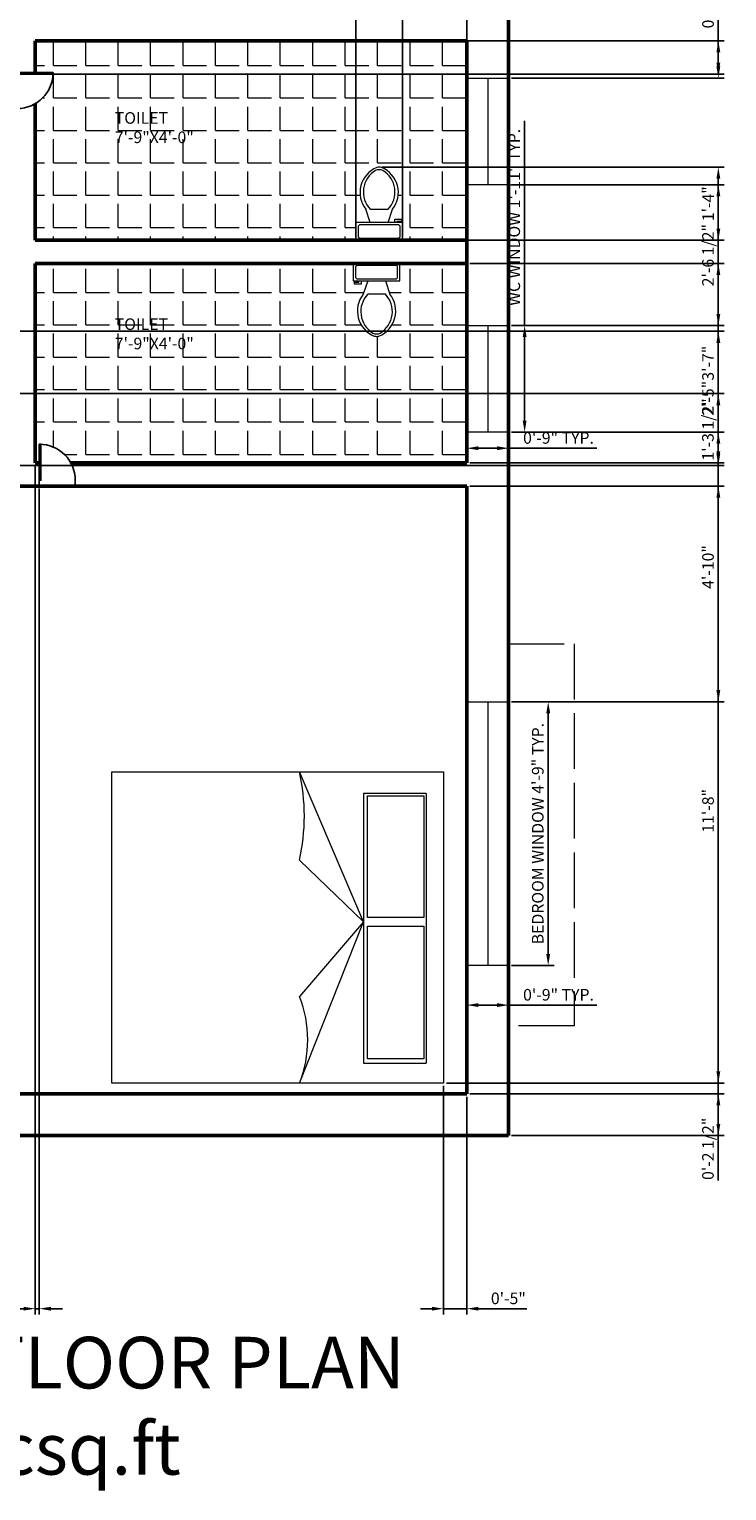
# Model space of a CAD drawing. Units: millimetres. Extents: x 3095 to 3505, y 1097 to 1734.
# Tile 3 of 5: x 3355 to 3505, y 1097 to 1412. Entities that reach past the tile are written whole.
import ezdxf

# ---------------------------------------------------------------- set-up
doc = ezdxf.new("R2010")
doc.units = ezdxf.units.MM
doc.linetypes.add('ACAD_ISO02W100', pattern=[15, 12, -3])
for name, color, linetype, lineweight, true_color in [('A-ANNO-DIMS', 32, 'Continuous', 18, 0xcd6928), ('A-ANNO-TEXT', 152, 'Continuous', 25, 0x2776bb), ('A-AREA-IDEN', 152, 'Continuous', 18, 0x2776bb), ('A-FLOR-FIXT', 9, 'Continuous', 18, 0xafd9aa), ('A-FLOR-PATT', 241, 'Continuous', 13, 0xf7abae), ('A-FURN', 9, 'Continuous', 18, 0xafd9aa), ('A-GLAZ', 9, 'Continuous', 18, 0xd19cc7), ('A-ROOF-OVHD', 152, 'ACAD_ISO02W100', 13, 0x2776bb)]:
    doc.layers.add(name, color=color, linetype=linetype, lineweight=lineweight, true_color=true_color)
doc.layers.add('A-DOOR', color=4, linetype='Continuous', lineweight=25)
doc.layers.add('A-WALL', color=7, linetype='Continuous', lineweight=50)
doc.styles.get("Standard").update_dxf_attribs({"font": 'arial.ttf'})
doc.dimstyles.new('ISO-25', dxfattribs={"dimtxt": 2.5, "dimasz": 2.5, "dimexe": 1.25, "dimexo": 0.625, "dimtad": 1, "dimlunit": 3, "dimtxsty": 'Standard', "dimcen": 2.5, "dimadec": 0, "dimazin": 0, "dimtfac": 1, "dimtmove": 0, "dimatfit": 3, "dimfxl": 1, "dimarcsym": 0})

# ---------------------------------------------------------------- blocks, each defined once
blk = doc.blocks.new('*U4')
for p, q in [((9.5, -6), (9.5, -2)), ((-10, -8.5), (-8, -8.5)), ((-10, -9.5), (-10, -8.5)), ((-7, -9.5), (-10, -9.5)), ((-8, -8.5), (-8, -8)), ((-7, -8), (-7, -9.5)), ((-4, -8), (-6, -14)), ((4, -8), (6, -14)), ((4, -14), (-4, -14))]:
    blk.add_line(p, q)
blk.add_lwpolyline([(10.5, -8), (10.5, 0), (-10.5, 0), (-10.5, -8)], close=True)
for points in [[(-9.5, -2), (-9.5, -6)], [(8.5, -1), (-8.5, -1)], [(-8.5, -7), (8.5, -7)]]:
    blk.add_lwpolyline(points)
for centre, radius, start, end in [((-8.62, -1.88), 0.884, 81.8699, 188.1301), ((-8.62, -6.12), 0.884, 171.8699, 278.1301), ((8.62, -1.88), 0.884, 351.8699, 98.1301), ((8.62, -6.12), 0.884, 261.8699, 8.1301), ((3.52, -21.58), 12.17, 141.46911, 247.97143), ((4.2, -21.82), 11.33, 136.36773, 238.94682), ((-3.52, -21.58), 12.17, 292.02843, 38.53071), ((-4.2, -21.82), 11.33, 301.05301, 43.63209), ((0, -27.88), 4, 245.73182, 294.26817), ((0, -29), 4, 254.86053, 285.13947)]:
    blk.add_arc(centre, radius, start, end)
blk = doc.blocks.new('*U8')
for p, q in [((0, 0), (0, -6)), ((40, 0), (40, -6))]:
    blk.add_line(p, q)
blk.add_lwpolyline([(0, 0), (0, 40), (1.75, 40), (1.75, 0)], close=True)
blk.add_arc((0, 0), 40, 0, 90)
blk = doc.blocks.new('*U6')
for p, q in [((0, 0), (0, -6)), ((40, 0), (40, -6))]:
    blk.add_line(p, q)
blk.add_lwpolyline([(0, 0), (0, 40), (1.75, 40), (1.75, 0)], close=True)
blk.add_arc((0, 0), 40, 0, 90)
blk = doc.blocks.new('BED-DOUBLE')
for p, q in [((4.67, 67.71), (4.67, 54.2)), ((4.67, 67.71), (62.81, 67.71)), ((62.81, 54.2), (62.81, 67.71)), ((32.4, 54.2), (0, 40.37)), ((4.67, 54.2), (62.81, 54.2)), ((32.4, 54.2), (19.1, 40.37)), ((67.13, 40.37), (32.4, 54.2)), ((32.4, 54.2), (48.47, 40.37))]:
    blk.add_line(p, q)
for points in [[(0, 71.42), (67.13, 71.42), (67.13, 0), (0, 0)], [(5.23, 67.2), (31.46, 67.2), (31.46, 55.05), (5.23, 55.05)], [(33.33, 67.2), (61.88, 67.2), (61.88, 55.05), (33.33, 55.05)]]:
    blk.add_lwpolyline(points, close=True)
for centre, radius, start, end in [((9.55, -1.59), 43.03, 77.1763, 102.8237), ((57.8, 17.19), 24.99, 68.0833, 111.9167)]:
    blk.add_arc(centre, radius, start, end)
blk = doc.blocks.new('WIN-BEDROOM')
for p, q in [((0, 56.87), (9, 56.87)), ((0, 0), (0, 56.87)), ((0, 56.87), (4.5, 56.87)), ((4.5, 56.87), (4.5, 0)), ((9, 56.87), (9, 0)), ((9, 0), (0, 0))]:
    blk.add_line(p, q)
blk = doc.blocks.new('WIN-TOILET')
for p, q in [((0, 23.01), (9, 23.01)), ((0, 0), (0, 23.01)), ((0, 23.01), (4.5, 23.01)), ((4.5, 23.01), (4.5, 0)), ((9, 23.01), (9, 0)), ((9, 0), (0, 0))]:
    blk.add_line(p, q)
blk = doc.blocks.new('*D20')
at = {"layer": 'A-ANNO-DIMS', "color": 0, "lineweight": -2, "transparency": 16777216}
for p, q in [((3458.49, 1266.84), (3467.64, 1266.84)), ((3466.39, 1212.47), (3466.39, 1264.34)), ((3458.49, 1209.97), (3467.64, 1209.97))]:
    blk.add_line(p, q, dxfattribs=at)
at = {"layer": 'A-ANNO-DIMS', "color": 0, "lineweight": 5, "transparency": 16777216}
for points in [[(3465.98, 1264.34), (3466.81, 1264.34), (3466.39, 1266.84)], [(3465.98, 1212.47), (3466.81, 1212.47), (3466.39, 1209.97)]]:
    blk.add_solid(points, dxfattribs=at)
at = {"layer": 'Defpoints', "color": 0, "lineweight": 5, "transparency": 16777216}
for p in [(3457.86, 1266.84), (3466.39, 1266.84), (3457.86, 1209.97)]:
    blk.add_point(p, dxfattribs=at)
at = {"layer": 'A-ANNO-DIMS', "color": 0, "transparency": 16777216, "insert": (3464.47, 1238.41), "char_height": 2.5, "attachment_point": 5, "rotation": 90}
blk.add_mtext('BEDROOM WINDOW 4\'-9" TYP.', dxfattribs=at)
blk = doc.blocks.new('*D21')
at = {"layer": 'A-ANNO-DIMS', "color": 0, "lineweight": -2, "transparency": 16777216}
for p, q in [((3448.86, 1209.35), (3448.86, 1200.19)), ((3457.86, 1209.35), (3457.86, 1200.19)), ((3451.36, 1201.44), (3455.36, 1201.44)), ((3457.86, 1201.44), (3476.85, 1201.44))]:
    blk.add_line(p, q, dxfattribs=at)
at = {"layer": 'A-ANNO-DIMS', "color": 0, "lineweight": 5, "transparency": 16777216}
for points in [[(3451.36, 1201.86), (3451.36, 1201.03), (3448.86, 1201.44)], [(3455.36, 1201.86), (3455.36, 1201.03), (3457.86, 1201.44)]]:
    blk.add_solid(points, dxfattribs=at)
at = {"layer": 'Defpoints', "color": 0, "lineweight": 5, "transparency": 16777216}
for p in [(3448.86, 1209.97), (3457.86, 1209.97), (3457.86, 1201.44)]:
    blk.add_point(p, dxfattribs=at)
at = {"layer": 'A-ANNO-DIMS', "color": 0, "transparency": 16777216, "insert": (3468.61, 1203.35), "char_height": 2.5, "attachment_point": 5}
blk.add_mtext('0\'-9" TYP.', dxfattribs=at)
blk = doc.blocks.new('*D22')
at = {"layer": 'A-ANNO-DIMS', "color": 0, "lineweight": -2, "transparency": 16777216}
for p, q in [((3461.31, 1347.95), (3461.31, 1392.07)), ((3458.49, 1347.95), (3462.56, 1347.95)), ((3461.31, 1327.44), (3461.31, 1345.45)), ((3458.49, 1324.94), (3462.56, 1324.94))]:
    blk.add_line(p, q, dxfattribs=at)
at = {"layer": 'A-ANNO-DIMS', "color": 0, "lineweight": 5, "transparency": 16777216}
for points in [[(3460.9, 1345.45), (3461.73, 1345.45), (3461.31, 1347.95)], [(3460.9, 1327.44), (3461.73, 1327.44), (3461.31, 1324.94)]]:
    blk.add_solid(points, dxfattribs=at)
at = {"layer": 'Defpoints', "color": 0, "lineweight": 5, "transparency": 16777216}
for p in [(3457.86, 1347.95), (3461.31, 1347.95), (3457.86, 1324.94)]:
    blk.add_point(p, dxfattribs=at)
at = {"layer": 'A-ANNO-DIMS', "color": 0, "transparency": 16777216, "insert": (3459.4, 1371.26), "char_height": 2.5, "attachment_point": 5, "rotation": 90}
blk.add_mtext('WC WINDOW 1\'-11" TYP.', dxfattribs=at)
blk = doc.blocks.new('*D23')
at = {"layer": 'A-ANNO-DIMS', "color": 0, "lineweight": -2, "transparency": 16777216}
for p, q in [((3448.86, 1324.32), (3448.86, 1320.24)), ((3457.86, 1324.32), (3457.86, 1320.24)), ((3451.36, 1321.49), (3455.36, 1321.49)), ((3457.86, 1321.49), (3476.85, 1321.49))]:
    blk.add_line(p, q, dxfattribs=at)
at = {"layer": 'A-ANNO-DIMS', "color": 0, "lineweight": 5, "transparency": 16777216}
for points in [[(3451.36, 1321.91), (3451.36, 1321.08), (3448.86, 1321.49)], [(3455.36, 1321.91), (3455.36, 1321.08), (3457.86, 1321.49)]]:
    blk.add_solid(points, dxfattribs=at)
at = {"layer": 'Defpoints', "color": 0, "lineweight": 5, "transparency": 16777216}
for p in [(3448.86, 1324.94), (3457.86, 1324.94), (3457.86, 1321.49)]:
    blk.add_point(p, dxfattribs=at)
at = {"layer": 'A-ANNO-DIMS', "color": 0, "transparency": 16777216, "insert": (3468.61, 1323.39), "char_height": 2.5, "attachment_point": 5}
blk.add_mtext('0\'-9" TYP.', dxfattribs=at)
blk = doc.blocks.new('*D40')
at = {"layer": 'A-ANNO-DIMS', "color": 0, "lineweight": -2, "transparency": 16777216}
for p, q in [((3458.49, 1454.16), (3504.29, 1454.16)), ((3503.04, 1451.66), (3503.04, 1403.79)), ((3458.49, 1401.29), (3504.29, 1401.29))]:
    blk.add_line(p, q, dxfattribs=at)
at = {"layer": 'A-ANNO-DIMS', "color": 0, "lineweight": 5, "transparency": 16777216}
for points in [[(3502.63, 1451.66), (3503.46, 1451.66), (3503.04, 1454.16)], [(3502.63, 1403.79), (3503.46, 1403.79), (3503.04, 1401.29)]]:
    blk.add_solid(points, dxfattribs=at)
at = {"layer": 'Defpoints', "color": 0, "lineweight": 5, "transparency": 16777216}
for p in [(3457.86, 1454.16), (3457.86, 1401.29), (3503.04, 1401.29)]:
    blk.add_point(p, dxfattribs=at)
at = {"layer": 'A-ANNO-DIMS', "color": 0, "transparency": 16777216, "insert": (3501.15, 1427.72), "char_height": 2.5, "attachment_point": 5, "rotation": 90}
blk.add_mtext('4\'-5"', dxfattribs=at)
blk = doc.blocks.new('*D41')
at = {"layer": 'A-ANNO-DIMS', "color": 0, "lineweight": -2, "transparency": 16777216}
for p, q in [((3458.49, 1378.28), (3504.29, 1378.28)), ((3503.04, 1375.78), (3503.04, 1350.45)), ((3458.49, 1347.95), (3504.29, 1347.95))]:
    blk.add_line(p, q, dxfattribs=at)
at = {"layer": 'A-ANNO-DIMS', "color": 0, "lineweight": 5, "transparency": 16777216}
for points in [[(3502.63, 1375.78), (3503.46, 1375.78), (3503.04, 1378.28)], [(3502.63, 1350.45), (3503.46, 1350.45), (3503.04, 1347.95)]]:
    blk.add_solid(points, dxfattribs=at)
at = {"layer": 'Defpoints', "color": 0, "lineweight": 5, "transparency": 16777216}
for p in [(3457.86, 1378.28), (3457.86, 1347.95), (3503.04, 1347.95)]:
    blk.add_point(p, dxfattribs=at)
at = {"layer": 'A-ANNO-DIMS', "color": 0, "transparency": 16777216, "insert": (3501.13, 1363.11), "char_height": 2.5, "attachment_point": 5, "rotation": 90}
blk.add_mtext('2\'-6 1/2"', dxfattribs=at)
blk = doc.blocks.new('*D42')
at = {"layer": 'A-ANNO-DIMS', "color": 0, "lineweight": -2, "transparency": 16777216}
for p, q in [((3458.49, 1324.94), (3504.29, 1324.94)), ((3503.04, 1322.44), (3503.04, 1269.34)), ((3458.49, 1266.84), (3504.29, 1266.84))]:
    blk.add_line(p, q, dxfattribs=at)
at = {"layer": 'A-ANNO-DIMS', "color": 0, "lineweight": 5, "transparency": 16777216}
for points in [[(3502.63, 1322.44), (3503.46, 1322.44), (3503.04, 1324.94)], [(3502.63, 1269.34), (3503.46, 1269.34), (3503.04, 1266.84)]]:
    blk.add_solid(points, dxfattribs=at)
at = {"layer": 'Defpoints', "color": 0, "lineweight": 5, "transparency": 16777216}
for p in [(3457.86, 1324.94), (3457.86, 1266.84), (3503.04, 1266.84)]:
    blk.add_point(p, dxfattribs=at)
at = {"layer": 'A-ANNO-DIMS', "color": 0, "transparency": 16777216, "insert": (3501.14, 1295.89), "char_height": 2.5, "attachment_point": 5, "rotation": 90}
blk.add_mtext('4\'-10"', dxfattribs=at)
blk = doc.blocks.new('*D46')
at = {"layer": 'A-ANNO-DIMS', "color": 0, "lineweight": -2, "transparency": 16777216}
for p, q in [((3449.49, 1313.32), (3504.29, 1313.32)), ((3503.04, 1310.82), (3503.04, 1175.82)), ((3458.49, 1173.32), (3504.29, 1173.32))]:
    blk.add_line(p, q, dxfattribs=at)
at = {"layer": 'A-ANNO-DIMS', "color": 0, "lineweight": 5, "transparency": 16777216}
for points in [[(3502.63, 1310.82), (3503.46, 1310.82), (3503.04, 1313.32)], [(3502.63, 1175.82), (3503.46, 1175.82), (3503.04, 1173.32)]]:
    blk.add_solid(points, dxfattribs=at)
at = {"layer": 'Defpoints', "color": 0, "lineweight": 5, "transparency": 16777216}
for p in [(3448.86, 1313.32), (3457.86, 1173.32), (3503.04, 1173.32)]:
    blk.add_point(p, dxfattribs=at)
at = {"layer": 'A-ANNO-DIMS', "color": 0, "transparency": 16777216, "insert": (3501.14, 1243.32), "char_height": 2.5, "attachment_point": 5, "rotation": 90}
blk.add_mtext('11\'-8"', dxfattribs=at)
blk = doc.blocks.new('*D47')
at = {"layer": 'A-ANNO-DIMS', "color": 0, "lineweight": -2, "transparency": 16777216}
for p, q in [((3449.49, 1361.32), (3504.29, 1361.32)), ((3503.04, 1320.82), (3503.04, 1358.82)), ((3449.49, 1318.32), (3504.29, 1318.32))]:
    blk.add_line(p, q, dxfattribs=at)
at = {"layer": 'A-ANNO-DIMS', "color": 0, "lineweight": 5, "transparency": 16777216}
for points in [[(3502.63, 1358.82), (3503.46, 1358.82), (3503.04, 1361.32)], [(3502.63, 1320.82), (3503.46, 1320.82), (3503.04, 1318.32)]]:
    blk.add_solid(points, dxfattribs=at)
at = {"layer": 'Defpoints', "color": 0, "lineweight": 5, "transparency": 16777216}
for p in [(3448.86, 1361.32), (3503.04, 1361.32), (3448.86, 1318.32)]:
    blk.add_point(p, dxfattribs=at)
at = {"layer": 'A-ANNO-DIMS', "color": 0, "transparency": 16777216, "insert": (3501.14, 1339.82), "char_height": 2.5, "attachment_point": 5, "rotation": 90}
blk.add_mtext('3\'-7"', dxfattribs=at)
blk = doc.blocks.new('*D59')
at = {"layer": 'A-ANNO-DIMS', "color": 0, "lineweight": -2, "transparency": 16777216}
for p, q in [((3424.96, 1366.94), (3424.96, 1729.27)), ((3427.46, 1728.02), (3432.49, 1728.02)), ((3434.99, 1366.94), (3434.99, 1729.27))]:
    blk.add_line(p, q, dxfattribs=at)
at = {"layer": 'A-ANNO-DIMS', "color": 0, "lineweight": 5, "transparency": 16777216}
for points in [[(3427.46, 1728.43), (3427.46, 1727.6), (3424.96, 1728.02)], [(3432.49, 1728.43), (3432.49, 1727.6), (3434.99, 1728.02)]]:
    blk.add_solid(points, dxfattribs=at)
at = {"layer": 'Defpoints', "color": 0, "lineweight": 5, "transparency": 16777216}
for p in [(3434.99, 1728.02), (3424.96, 1366.32), (3434.99, 1366.32)]:
    blk.add_point(p, dxfattribs=at)
at = {"layer": 'A-ANNO-DIMS', "color": 0, "transparency": 16777216, "insert": (3429.98, 1729.92), "char_height": 2.5, "attachment_point": 5}
blk.add_mtext('0\'-10"', dxfattribs=at)
blk = doc.blocks.new('*D60')
at = {"layer": 'A-ANNO-DIMS', "color": 0, "lineweight": -2, "transparency": 16777216}
for p, q in [((3430.6, 1382.07), (3504.29, 1382.07)), ((3503.04, 1368.82), (3503.04, 1379.57)), ((3435.62, 1366.32), (3504.29, 1366.32))]:
    blk.add_line(p, q, dxfattribs=at)
at = {"layer": 'A-ANNO-DIMS', "color": 0, "lineweight": 5, "transparency": 16777216}
for points in [[(3502.63, 1379.57), (3503.46, 1379.57), (3503.04, 1382.07)], [(3502.63, 1368.82), (3503.46, 1368.82), (3503.04, 1366.32)]]:
    blk.add_solid(points, dxfattribs=at)
at = {"layer": 'Defpoints', "color": 0, "lineweight": 5, "transparency": 16777216}
for p in [(3429.98, 1382.07), (3503.04, 1382.07), (3434.99, 1366.32)]:
    blk.add_point(p, dxfattribs=at)
at = {"layer": 'A-ANNO-DIMS', "color": 0, "transparency": 16777216, "insert": (3501.16, 1374.2), "char_height": 2.5, "attachment_point": 5, "rotation": 90}
blk.add_mtext('1\'-4"', dxfattribs=at)
blk = doc.blocks.new('*D61')
at = {"layer": 'A-ANNO-DIMS', "color": 0, "lineweight": -2, "transparency": 16777216}
for p, q in [((3434.99, 1366.94), (3434.99, 1729.27)), ((3437.49, 1728.02), (3446.36, 1728.02)), ((3448.86, 1366.94), (3448.86, 1729.27))]:
    blk.add_line(p, q, dxfattribs=at)
at = {"layer": 'A-ANNO-DIMS', "color": 0, "lineweight": 5, "transparency": 16777216}
for points in [[(3437.49, 1728.43), (3437.49, 1727.6), (3434.99, 1728.02)], [(3446.36, 1728.43), (3446.36, 1727.6), (3448.86, 1728.02)]]:
    blk.add_solid(points, dxfattribs=at)
at = {"layer": 'Defpoints', "color": 0, "lineweight": 5, "transparency": 16777216}
for p in [(3448.86, 1728.02), (3434.99, 1366.32), (3448.86, 1366.32)]:
    blk.add_point(p, dxfattribs=at)
at = {"layer": 'A-ANNO-DIMS', "color": 0, "transparency": 16777216, "insert": (3441.93, 1729.9), "char_height": 2.5, "attachment_point": 5}
blk.add_mtext('1\'-2"', dxfattribs=at)
blk = doc.blocks.new('*D63')
at = {"layer": 'A-ANNO-DIMS', "color": 0, "lineweight": -2, "transparency": 16777216}
for p, q in [((3503.04, 1409.32), (3503.04, 1419.71)), ((3356.49, 1409.32), (3504.29, 1409.32)), ((3503.04, 1404.64), (3503.04, 1406.82)), ((3356.49, 1402.14), (3504.29, 1402.14))]:
    blk.add_line(p, q, dxfattribs=at)
at = {"layer": 'A-ANNO-DIMS', "color": 0, "lineweight": 5, "transparency": 16777216}
for points in [[(3502.63, 1406.82), (3503.46, 1406.82), (3503.04, 1409.32)], [(3502.63, 1404.64), (3503.46, 1404.64), (3503.04, 1402.14)]]:
    blk.add_solid(points, dxfattribs=at)
at = {"layer": 'Defpoints', "color": 0, "lineweight": 5, "transparency": 16777216}
for p in [(3355.86, 1409.32), (3503.04, 1409.32), (3355.86, 1402.14)]:
    blk.add_point(p, dxfattribs=at)
at = {"layer": 'A-ANNO-DIMS', "color": 0, "transparency": 16777216, "insert": (3501.14, 1415.76), "char_height": 2.5, "attachment_point": 5, "rotation": 90}
blk.add_mtext('0\'-7"', dxfattribs=at)
blk = doc.blocks.new('*D64')
at = {"layer": 'A-ANNO-DIMS', "color": 0, "lineweight": -2, "transparency": 16777216}
for p, q in [((3355.86, 1317.69), (3355.86, 1134.75)), ((3356.76, 1312.81), (3356.76, 1134.75)), ((3353.36, 1136), (3342.97, 1136)), ((3356.76, 1136), (3355.86, 1136)), ((3359.26, 1136), (3361.76, 1136))]:
    blk.add_line(p, q, dxfattribs=at)
at = {"layer": 'A-ANNO-DIMS', "color": 0, "lineweight": 5, "transparency": 16777216}
for points in [[(3353.36, 1136.41), (3353.36, 1135.58), (3355.86, 1136)], [(3359.26, 1136.41), (3359.26, 1135.58), (3356.76, 1136)]]:
    blk.add_solid(points, dxfattribs=at)
at = {"layer": 'Defpoints', "color": 0, "lineweight": 5, "transparency": 16777216}
for p in [(3355.86, 1318.32), (3356.76, 1313.43), (3355.86, 1136)]:
    blk.add_point(p, dxfattribs=at)
at = {"layer": 'A-ANNO-DIMS', "color": 0, "transparency": 16777216, "insert": (3346.91, 1137.9), "char_height": 2.5, "attachment_point": 5}
blk.add_mtext('0\'-1"', dxfattribs=at)
blk = doc.blocks.new('*D69')
at = {"layer": 'A-ANNO-DIMS', "color": 0, "lineweight": -2, "transparency": 16777216}
for p, q in [((3250.48, 1333.27), (3504.29, 1333.27)), ((3503.04, 1330.77), (3503.04, 1320.3)), ((3250.48, 1317.8), (3504.29, 1317.8))]:
    blk.add_line(p, q, dxfattribs=at)
at = {"layer": 'A-ANNO-DIMS', "color": 0, "lineweight": 5, "transparency": 16777216}
for points in [[(3502.63, 1330.77), (3503.46, 1330.77), (3503.04, 1333.27)], [(3502.63, 1320.3), (3503.46, 1320.3), (3503.04, 1317.8)]]:
    blk.add_solid(points, dxfattribs=at)
at = {"layer": 'Defpoints', "color": 0, "lineweight": 5, "transparency": 16777216}
for p in [(3249.85, 1333.27), (3249.85, 1317.8), (3503.04, 1317.8)]:
    blk.add_point(p, dxfattribs=at)
at = {"layer": 'A-ANNO-DIMS', "color": 0, "transparency": 16777216, "insert": (3501.12, 1325.54), "char_height": 2.5, "attachment_point": 5, "rotation": 90}
blk.add_mtext('1\'-3 1/2"', dxfattribs=at)
blk = doc.blocks.new('*D77')
at = {"layer": 'A-ANNO-DIMS', "color": 0, "lineweight": -2, "transparency": 16777216}
for p, q in [((3194.49, 1346.71), (3504.29, 1346.71)), ((3503.04, 1344.21), (3503.04, 1320.3)), ((3250.48, 1317.8), (3504.29, 1317.8))]:
    blk.add_line(p, q, dxfattribs=at)
at = {"layer": 'A-ANNO-DIMS', "color": 0, "lineweight": 5, "transparency": 16777216}
for points in [[(3502.63, 1344.21), (3503.46, 1344.21), (3503.04, 1346.71)], [(3502.63, 1320.3), (3503.46, 1320.3), (3503.04, 1317.8)]]:
    blk.add_solid(points, dxfattribs=at)
at = {"layer": 'Defpoints', "color": 0, "lineweight": 5, "transparency": 16777216}
for p in [(3193.86, 1346.71), (3249.85, 1317.8), (3503.04, 1317.8)]:
    blk.add_point(p, dxfattribs=at)
at = {"layer": 'A-ANNO-DIMS', "color": 0, "transparency": 16777216, "insert": (3501.14, 1332.26), "char_height": 2.5, "attachment_point": 5, "rotation": 90}
blk.add_mtext('2\'-5"', dxfattribs=at)
blk = doc.blocks.new('*D86')
at = {"layer": 'A-ANNO-DIMS', "color": 0, "lineweight": -2, "transparency": 16777216}
for p, q in [((3503.04, 1187.14), (3503.04, 1189.64)), ((3444.47, 1184.64), (3504.29, 1184.64)), ((3449.49, 1182.32), (3504.29, 1182.32)), ((3503.04, 1184.64), (3503.04, 1182.32)), ((3503.04, 1179.82), (3503.04, 1163.6))]:
    blk.add_line(p, q, dxfattribs=at)
at = {"layer": 'A-ANNO-DIMS', "color": 0, "lineweight": 5, "transparency": 16777216}
for points in [[(3502.63, 1187.14), (3503.46, 1187.14), (3503.04, 1184.64)], [(3502.63, 1179.82), (3503.46, 1179.82), (3503.04, 1182.32)]]:
    blk.add_solid(points, dxfattribs=at)
at = {"layer": 'Defpoints', "color": 0, "lineweight": 5, "transparency": 16777216}
for p in [(3443.85, 1184.64), (3448.86, 1182.32), (3503.04, 1182.32)]:
    blk.add_point(p, dxfattribs=at)
at = {"layer": 'A-ANNO-DIMS', "color": 0, "transparency": 16777216, "insert": (3501.13, 1170.46), "char_height": 2.5, "attachment_point": 5, "rotation": 90}
blk.add_mtext('0\'-2 1/2"', dxfattribs=at)
blk = doc.blocks.new('*D87')
at = {"layer": 'A-ANNO-DIMS', "color": 0, "lineweight": -2, "transparency": 16777216}
for p, q in [((3443.85, 1184.01), (3443.85, 1134.75)), ((3448.86, 1181.69), (3448.86, 1134.75)), ((3441.35, 1136), (3438.85, 1136)), ((3443.85, 1136), (3448.86, 1136)), ((3451.36, 1136), (3461.76, 1136))]:
    blk.add_line(p, q, dxfattribs=at)
at = {"layer": 'A-ANNO-DIMS', "color": 0, "lineweight": 5, "transparency": 16777216}
for points in [[(3441.35, 1136.41), (3441.35, 1135.58), (3443.85, 1136)], [(3451.36, 1136.41), (3451.36, 1135.58), (3448.86, 1136)]]:
    blk.add_solid(points, dxfattribs=at)
at = {"layer": 'Defpoints', "color": 0, "lineweight": 5, "transparency": 16777216}
for p in [(3443.85, 1184.64), (3448.86, 1182.32), (3448.86, 1136)]:
    blk.add_point(p, dxfattribs=at)
at = {"layer": 'A-ANNO-DIMS', "color": 0, "transparency": 16777216, "insert": (3457.81, 1137.9), "char_height": 2.5, "attachment_point": 5}
blk.add_mtext('0\'-5"', dxfattribs=at)

msp = doc.modelspace()

# ---------------------------------------------------------------- hatches: boundary and pattern name
at = {"layer": 'A-FLOR-PATT'}
h = msp.add_hatch(dxfattribs=at)
h.set_pattern_fill('ANGLE', color=256)
h.set_pattern_definition([(0, (0, 0), (0, 6.985), [5.08, -1.905]), (90, (0, 0), (-6.985, 4e-16), [5.08, -1.905])])
h.paths.add_polyline_path([(3311.862, 1668.316), (3273.923, 1668.316), (3273.923, 1664.496), (3270.819, 1664.496), (3271.774, 1661.631, -0.5301431), (3268.909, 1652.448, -0.530136), (3266.044, 1661.631), (3266.999, 1664.496), (3265.566, 1664.496), (3265.566, 1663.78), (3264.134, 1663.78), (3264.134, 1664.496), (3263.895, 1664.496), (3263.895, 1668.316), (3258.862, 1668.316), (3258.862, 1527.316), (3311.862, 1527.316), (3311.862, 1534.492), (3307.983, 1534.492), (3307.983, 1534.831), (3307.991, 1534.831, -0.2562565), (3311.862, 1541.211)])
h.paths.add_polyline_path([(3448.862, 1409.316), (3355.862, 1409.316), (3355.862, 1402.478), (3359.742, 1402.478), (3359.742, 1402.139), (3359.734, 1402.139, -0.2562565), (3355.862, 1395.759), (3355.862, 1366.316), (3424.964, 1366.316), (3424.964, 1370.136), (3428.068, 1370.136), (3427.113, 1373.001, -0.4652664), (3428.865, 1381.717, -0.3212229), (3431.09, 1381.717, -0.4652592), (3432.843, 1373.001), (3431.888, 1370.136), (3433.32, 1370.136), (3433.32, 1370.853), (3434.753, 1370.853), (3434.992, 1370.136), (3434.992, 1366.316), (3448.862, 1366.316)])
h.paths.add_polyline_path([(3428.308, 1345.964, -0.4652592), (3426.555, 1354.679), (3427.51, 1357.544), (3426.078, 1357.544), (3426.078, 1356.828), (3424.645, 1356.828), (3424.407, 1357.544), (3424.407, 1361.316), (3355.862, 1361.316), (3355.862, 1322.305, -0.0398063), (3357.095, 1322.349), (3357.095, 1322.357), (3356.756, 1322.357, -0.2743513), (3363.565, 1318.316), (3448.862, 1318.316), (3448.862, 1361.316), (3434.434, 1361.316), (3434.434, 1357.544), (3431.331, 1357.544), (3432.286, 1354.679, -0.4652664), (3430.533, 1345.964, -0.3212229)])

# ---------------------------------------------------------------- linework, layer by layer
at = {"layer": 'A-ROOF-OVHD'}
for p, q in [((3457.862, 1279.358), (3471.993, 1279.358)), ((3471.993, 1279.358), (3471.993, 1196.994)), ((3471.993, 1196.994), (3457.862, 1196.994))]:
    msp.add_line(p, q, dxfattribs=at)
at = {"layer": 'A-WALL'}
for p, q in [((3457.862, 1677.316), (3457.862, 1173.316)), ((3355.862, 1409.316), (3355.862, 1402.139)), ((3355.862, 1409.316), (3448.862, 1409.316)), ((3448.862, 1409.316), (3448.862, 1318.316)), ((3355.862, 1395.759), (3355.862, 1366.316)), ((3355.862, 1366.316), (3448.862, 1366.316)), ((3355.862, 1361.316), (3448.862, 1361.316)), ((3355.862, 1361.316), (3355.862, 1318.316)), ((3355.862, 1318.316), (3357.095, 1318.316)), ((3363.565, 1318.316), (3448.862, 1318.316)), ((3316.862, 1313.316), (3448.862, 1313.316)), ((3448.862, 1313.316), (3448.862, 1182.316)), ((3448.862, 1182.316), (3316.862, 1182.316)), ((3457.862, 1173.316), (3145.862, 1173.316))]:
    msp.add_line(p, q, dxfattribs=at)

# ---------------------------------------------------------------- block references
at = {"layer": 'A-DOOR', "xscale": 0.1939559161486229, "yscale": 0.1939559161486229, "zscale": 0.1939559161486229, "rotation": 270}
msp.add_blockref('*U8', (3351.983, 1402.478), dxfattribs=at)
at = {"layer": 'A-DOOR', "xscale": 0.1939559161486229, "yscale": 0.1939559161486229, "zscale": 0.1939559161486229}
msp.add_blockref('*U6', (3356.756, 1314.598), dxfattribs=at)
at = {"layer": 'A-FLOR-FIXT', "xscale": 0.4775205747460847, "yscale": 0.4775205747460847, "zscale": 0.4775205747460847, "rotation": 180.0000000000001}
msp.add_blockref('*U4', (3429.978, 1366.316), dxfattribs=at)
at = {"layer": 'A-FLOR-FIXT', "xscale": 0.4775205747460847, "yscale": 0.4775205747460847, "zscale": 0.4775205747460847}
msp.add_blockref('*U4', (3429.421, 1361.365), dxfattribs=at)
at = {"layer": 'A-FURN', "rotation": 270.0000000000006}
msp.add_blockref('BED-DOUBLE', (3372.422, 1251.764), dxfattribs=at)
at = {"layer": 'A-GLAZ'}
for name, p in [('WIN-TOILET', (3448.862, 1378.277)), ('WIN-TOILET', (3448.862, 1324.943)), ('WIN-BEDROOM', (3448.862, 1209.974))]:
    msp.add_blockref(name, p, dxfattribs=at)

# ---------------------------------------------------------------- texts
at = {"layer": 'A-ANNO-TEXT', "insert": (3277.968, 1129.938), "char_height": 11.14035, "attachment_point": 1}
msp.add_mtext_dynamic_manual_height_columns('GROUND FLOOR PLAN\\PArea:1092csq.ft', width=1117.06792, gutter_width=55.702, heights=[0], dxfattribs=at)
at = {"layer": 'A-AREA-IDEN', "char_height": 2.5, "attachment_point": 1}
for insert in [(3373.024, 1393.938), (3373.024, 1349.482)]:
    msp.add_mtext_dynamic_manual_height_columns('TOILET \\P7\'-9"X4\'-0"', width=29.88449, gutter_width=12.5, heights=[0], dxfattribs=dict(at, insert=insert))

# ---------------------------------------------------------------- dimensions: what is measured, and where the dimension line sits
at = {"layer": 'A-ANNO-DIMS'}
for base, p1, p2, picture, middle in [((3434.992, 1728.017), (3424.964, 1366.316), (3434.992, 1366.316), '*D59', (3429.978, 1729.919)), ((3448.862, 1728.017), (3434.992, 1366.316), (3448.862, 1366.316), '*D61', (3441.927, 1729.897)), ((3355.862, 1135.996), (3356.756, 1313.435), (3355.862, 1318.316), '*D64', (3346.915, 1137.898)), ((3448.862, 1135.996), (3443.846, 1184.638), (3448.862, 1182.316), '*D87', (3457.81, 1137.898))]:
    dim = msp.add_linear_dim(base=base, p1=p1, p2=p2, dimstyle='ISO-25', override={"dimdec": 1, "dimlfac": 1, "dimrnd": 0, "dimzin": 1, "dimdsep": 46, "dimlunit": 4, "dimfrac": 2}, dxfattribs=at)
    dim.commit()
    dim.dimension.update_dxf_attribs({"geometry": picture, "text_midpoint": middle})
for base, p1, p2, picture, middle in [((3503.043, 1401.286), (3457.862, 1454.161), (3457.862, 1401.286), '*D40', (3501.147, 1427.723)), ((3503.043, 1409.316), (3355.862, 1402.139), (3355.862, 1409.316), '*D63', (3501.141, 1415.764)), ((3503.043, 1382.074), (3434.992, 1366.316), (3429.978, 1382.074), '*D60', (3501.163, 1374.195)), ((3503.043, 1347.952), (3457.862, 1378.277), (3457.862, 1347.952), '*D41', (3501.125, 1363.115)), ((3503.043, 1361.316), (3448.862, 1318.316), (3448.862, 1361.316), '*D47', (3501.141, 1339.816)), ((3503.043, 1317.802), (3193.862, 1346.711), (3249.851, 1317.802), '*D77', (3501.141, 1332.256)), ((3503.043, 1317.802), (3249.851, 1333.27), (3249.851, 1317.802), '*D69', (3501.124, 1325.536)), ((3503.043, 1266.84), (3457.862, 1324.943), (3457.862, 1266.84), '*D42', (3501.141, 1295.892)), ((3503.043, 1173.316), (3448.862, 1313.316), (3457.862, 1173.316), '*D46', (3501.141, 1243.316)), ((3503.043, 1182.316), (3443.846, 1184.638), (3448.862, 1182.316), '*D86', (3501.125, 1170.456))]:
    dim = msp.add_linear_dim(base=base, p1=p1, p2=p2, angle=90, dimstyle='ISO-25', override={"dimdec": 1, "dimlfac": 1, "dimrnd": 0, "dimzin": 1, "dimdsep": 46, "dimlunit": 4, "dimfrac": 2}, dxfattribs=at)
    dim.commit()
    dim.dimension.update_dxf_attribs({"geometry": picture, "text_midpoint": middle})
for base, p1, p2, text, picture, middle in [((3461.314, 1347.952), (3457.862, 1324.943), (3457.862, 1347.952), 'WC WINDOW <> TYP.', '*D22', (3459.395, 1371.26)), ((3466.392, 1266.84), (3457.862, 1209.974), (3457.862, 1266.84), 'BEDROOM WINDOW <> TYP.', '*D20', (3464.474, 1238.407))]:
    dim = msp.add_linear_dim(base=base, p1=p1, p2=p2, angle=90, text=text, dimstyle='ISO-25', override={"dimdec": 1, "dimlfac": 1, "dimrnd": 0, "dimzin": 1, "dimdsep": 46, "dimlunit": 4, "dimfrac": 2}, dxfattribs=at)
    dim.commit()
    dim.dimension.update_dxf_attribs({"geometry": picture, "text_midpoint": middle})
for base, p1, p2, picture, middle in [((3457.862, 1321.492), (3448.862, 1324.943), (3457.862, 1324.943), '*D23', (3468.607, 1323.393)), ((3457.862, 1201.444), (3448.862, 1209.974), (3457.862, 1209.974), '*D21', (3468.607, 1203.346))]:
    dim = msp.add_linear_dim(base=base, p1=p1, p2=p2, text='<> TYP.', dimstyle='ISO-25', override={"dimdec": 1, "dimlfac": 1, "dimrnd": 0, "dimzin": 1, "dimdsep": 46, "dimlunit": 4, "dimfrac": 2}, dxfattribs=at)
    dim.commit()
    dim.dimension.update_dxf_attribs({"geometry": picture, "text_midpoint": middle})

doc.saveas('drawing.dxf')
